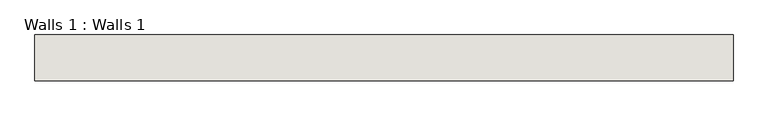
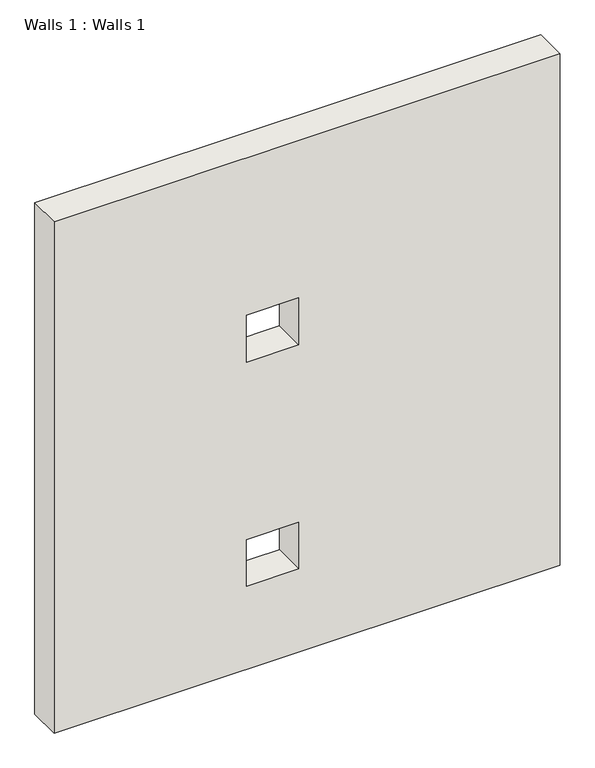
"""IFC4 building model written with IfcOpenShell, lengths in millimetres: wall geometry, Walls 1 : Walls 1."""

from ifc_helpers import new_model, si_unit, frame, origin, place, context, project, spatial, polyline, outline, extrude, source, transform, mapped, element, save


def walls_1_walls_1_ac0e2196(model_context):
    return source(origin(), model_context, "Body", "SweptSolid", [
        extrude(outline(polyline([(14096.0, -4690.01982), (14096.0, -17890.01982), (0.0, -17890.01982), (0.0, -4690.01982), (14096.0, -4690.01982)]), holes=[polyline([(3574.5396593, -11506.4727104), (2294.5396593, -11506.4727104), (2294.5396593, -12866.4727104), (3574.5396593, -12866.4727104), (3574.5396593, -11506.4727104)]), polyline([(9764.2267958, -11506.4727104), (8462.0666166, -11506.4727104), (8462.0666166, -12866.4727104), (9764.2267958, -12866.4727104), (9764.2267958, -11506.4727104)])]), frame((0.0, -8799.4475106, 0.0), z_axis=(0.0, 1.0, 0.0), x_axis=(0.0, 0.0, 1.0)), (0.0, 0.0, 1.0), 866.550948),
    ])


if __name__ == "__main__":
    model = new_model("IFC4")
    model_context = context("Model", 3, world=origin())
    ifc_project = project(units=[si_unit("LENGTHUNIT", "METRE", prefix="MILLI")], contexts=[model_context])
    site = spatial("IfcSite", under=ifc_project)
    building = spatial("IfcBuilding", under=site)
    placement = place(None, origin())
    walls_1_walls_1_shape = walls_1_walls_1_ac0e2196(model_context)
    element("IfcWall", 1, ObjectType="Walls 1 : Walls 1", at=placement, inside=building, context=model_context, shape_type="MappedRepresentation", body=[
        mapped(walls_1_walls_1_shape, transform((0.0, 0.0, 0.0), x_axis=(1.0, 0.0, 0.0), y_axis=(0.0, 1.0, 0.0), z_axis=(0.0, 0.0, 1.0))),
    ])
    save(model, "model.ifc")

# Revit data of these elements
# Element 1 (IfcWall, "Walls 1 : Walls 1")
#   Materials on its faces: "Default Wall"
# Materials
#   "Default Wall": colour RGB 80 80 80, transparency 0
